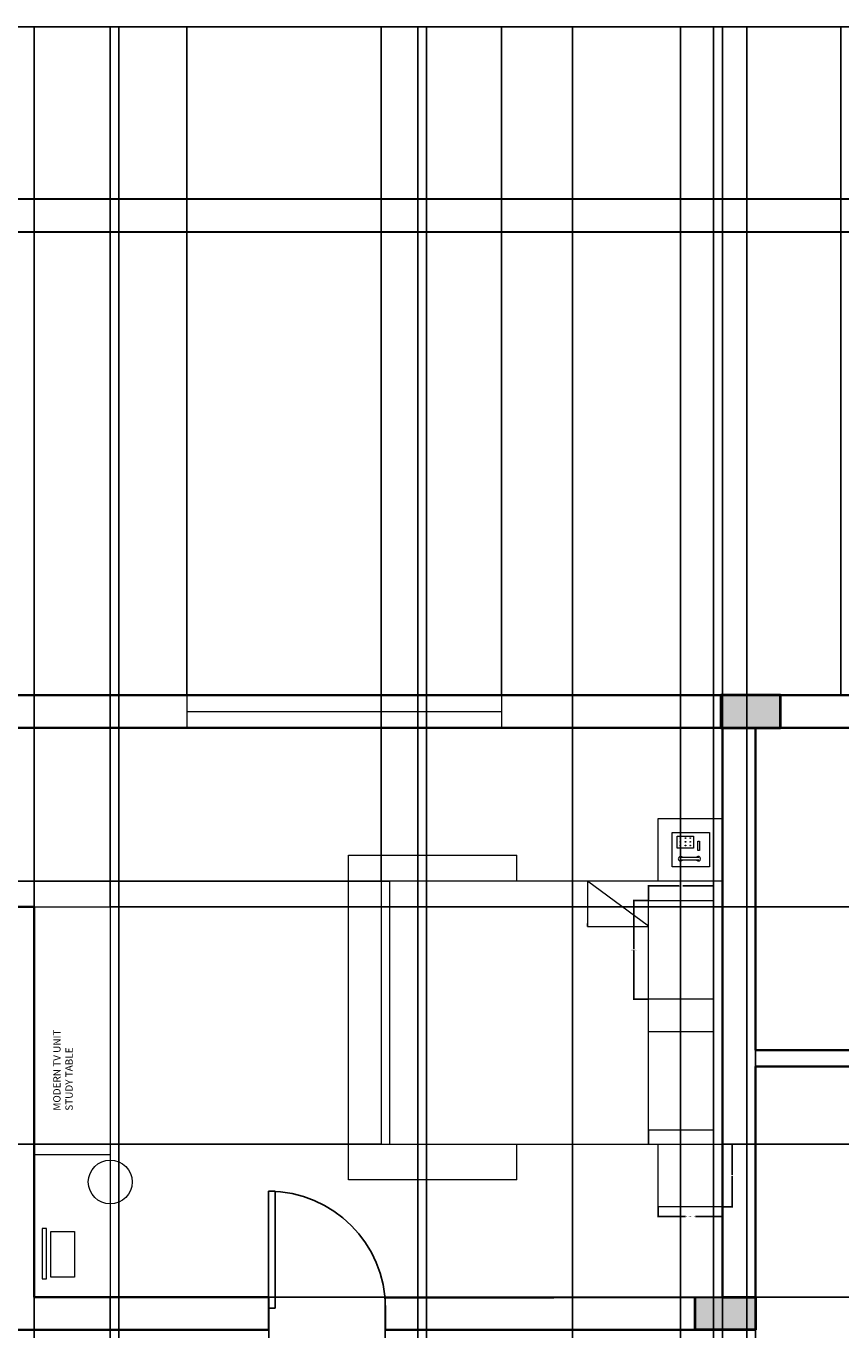
# Model space of a CAD drawing. Units: inches. Extents: x 1210 to 1836, y 84 to 1122.
# Tile 4 of 5: x 1353 to 1576, y 764 to 1122. Entities that reach past the tile are written whole.
import ezdxf

# ---------------------------------------------------------------- set-up
doc = ezdxf.new("R2010")
doc.units = ezdxf.units.IN
doc.header["$MEASUREMENT"] = 0
for name, color, linetype, lineweight in [('A-ANNO-DIMS', 2, 'Continuous', 18), ('A-ANNO-TEXT', 7, 'Continuous', 18), ('A-COLS', 7, 'Continuous', 40), ('A-COLS-PATT', 6, 'Continuous', 13), ('A-EQPM', 8, 'Continuous', 13), ('A-FURN', 9, 'Continuous', 18), ('A-FURN-FIXD', 32, 'Continuous', 18), ('A-GLAZ', 4, 'Continuous', 18), ('A-WALL', 7, 'Continuous', 35), ('C-PROP', 32, 'Continuous', 30), ('DOORS', 24, 'Continuous', 25)]:
    doc.layers.add(name, color=color, linetype=linetype, lineweight=lineweight)
doc.styles.get("Standard").update_dxf_attribs({"font": 'arial.ttf'})
doc.dimstyles.get("Standard").update_dxf_attribs({"dimtxt": 0.18, "dimasz": 0.18, "dimexe": 0.18, "dimexo": 0.0625, "dimgap": 0.09, "dimtad": 0, "dimtih": 1, "dimtoh": 1, "dimdec": 4, "dimzin": 0, "dimdsep": 46, "dimtxsty": 'Standard', "dimcen": 0.09, "dimadec": 0, "dimazin": 0, "dimtfac": 1, "dimtdec": 4, "dimtofl": 0, "dimtmove": 0, "dimatfit": 3, "dimfxl": 1, "dimtolj": 1, "dimtzin": 0, "dimarcsym": 0})

# ---------------------------------------------------------------- blocks, each defined once
blk = doc.blocks.new('*U6')
for p, q in [((0, 0), (0, -6)), ((32, 0), (32, -6))]:
    blk.add_line(p, q)
blk.add_lwpolyline([(0, 0), (0, 32), (1.75, 32), (1.75, 0)], close=True)
blk.add_arc((0, 0), 32, 0, 90)
blk = doc.blocks.new('PILLOW')
blk.add_lwpolyline([(0, 27), (17.76, 27), (17.76, 0), (0, 0)], close=True)
blk = doc.blocks.new('NIGHTSTAND')
blk.add_lwpolyline([(0, 17.21), (17.61, 17.21), (17.61, 0), (0, 0)], close=True)
blk = doc.blocks.new('STOOL-ROUND')
blk.add_circle((6, 6), 6)
blk = doc.blocks.new('*D16')
at = {"layer": 'A-ANNO-DIMS', "color": 0, "lineweight": -2, "transparency": 16777216}
for p, q in [((1522.97, 881.87), (1518.8, 881.87)), ((1518.98, 881.69), (1518.98, 868.55)), ((1518.98, 855.05), (1518.98, 868.19)), ((1522.97, 854.87), (1518.8, 854.87))]:
    blk.add_line(p, q, dxfattribs=at)
at = {"layer": 'A-ANNO-DIMS', "color": 0, "transparency": 16777216}
for points in [[(1518.95, 881.69), (1519.01, 881.69), (1518.98, 881.87)], [(1518.95, 855.05), (1519.01, 855.05), (1518.98, 854.87)]]:
    blk.add_solid(points, dxfattribs=at)
at = {"layer": 'Defpoints', "color": 0, "transparency": 16777216}
for p in [(1518.98, 881.87), (1523.03, 881.87), (1523.03, 854.87)]:
    blk.add_point(p, dxfattribs=at)
at = {"layer": 'A-ANNO-DIMS', "color": 0, "transparency": 16777216, "insert": (1518.98, 868.37), "char_height": 0.18, "attachment_point": 5}
blk.add_mtext('\\A1;PILLOW 27 TYP.', dxfattribs=at)
blk = doc.blocks.new('*D17')
at = {"layer": 'A-ANNO-DIMS', "color": 0, "lineweight": -2, "transparency": 16777216}
for p, q in [((1523.03, 881.93), (1523.03, 886.1)), ((1523.21, 885.92), (1531.4, 885.92)), ((1540.62, 885.92), (1532.43, 885.92)), ((1540.8, 881.93), (1540.8, 886.1))]:
    blk.add_line(p, q, dxfattribs=at)
at = {"layer": 'A-ANNO-DIMS', "color": 0, "transparency": 16777216}
for points in [[(1523.21, 885.95), (1523.21, 885.89), (1523.03, 885.92)], [(1540.62, 885.95), (1540.62, 885.89), (1540.8, 885.92)]]:
    blk.add_solid(points, dxfattribs=at)
at = {"layer": 'Defpoints', "color": 0, "transparency": 16777216}
for p in [(1540.8, 885.92), (1523.03, 881.87), (1540.8, 881.87)]:
    blk.add_point(p, dxfattribs=at)
at = {"layer": 'A-ANNO-DIMS', "color": 0, "transparency": 16777216, "insert": (1531.92, 885.92), "char_height": 0.18, "attachment_point": 5}
blk.add_mtext('\\A1;18 TYP.', dxfattribs=at)
blk = doc.blocks.new('*D18')
at = {"layer": 'A-ANNO-DIMS', "color": 0, "lineweight": -2, "transparency": 16777216}
for p, q in [((1525.71, 797.84), (1525.71, 795.08)), ((1543.32, 797.84), (1543.32, 795.08)), ((1525.89, 795.26), (1533.14, 795.26)), ((1543.14, 795.26), (1535.89, 795.26))]:
    blk.add_line(p, q, dxfattribs=at)
at = {"layer": 'A-ANNO-DIMS', "color": 0, "transparency": 16777216}
for points in [[(1525.89, 795.29), (1525.89, 795.23), (1525.71, 795.26)], [(1543.14, 795.29), (1543.14, 795.23), (1543.32, 795.26)]]:
    blk.add_solid(points, dxfattribs=at)
at = {"layer": 'Defpoints', "color": 0, "transparency": 16777216}
for p in [(1525.71, 797.91), (1543.32, 797.91), (1543.32, 795.26)]:
    blk.add_point(p, dxfattribs=at)
at = {"layer": 'A-ANNO-DIMS', "color": 0, "transparency": 16777216, "insert": (1534.52, 795.26), "char_height": 0.18, "attachment_point": 5}
blk.add_mtext('\\A1;NIGHTSTAND 18 TYP.', dxfattribs=at)
blk = doc.blocks.new('*D19')
at = {"layer": 'A-ANNO-DIMS', "color": 0, "lineweight": -2, "transparency": 16777216}
for p, q in [((1543.39, 815.12), (1546.15, 815.12)), ((1545.97, 814.94), (1545.97, 806.69)), ((1545.97, 798.09), (1545.97, 806.33)), ((1543.39, 797.91), (1546.15, 797.91))]:
    blk.add_line(p, q, dxfattribs=at)
at = {"layer": 'A-ANNO-DIMS', "color": 0, "transparency": 16777216}
for points in [[(1545.94, 814.94), (1546, 814.94), (1545.97, 815.12)], [(1545.94, 798.09), (1546, 798.09), (1545.97, 797.91)]]:
    blk.add_solid(points, dxfattribs=at)
at = {"layer": 'Defpoints', "color": 0, "transparency": 16777216}
for p in [(1543.32, 815.12), (1545.97, 815.12), (1543.32, 797.91)]:
    blk.add_point(p, dxfattribs=at)
at = {"layer": 'A-ANNO-DIMS', "color": 0, "transparency": 16777216, "insert": (1545.97, 806.51), "char_height": 0.18, "attachment_point": 5}
blk.add_mtext('\\A1;17 TYP.', dxfattribs=at)
blk = doc.blocks.new('*D22')
at = {"layer": 'A-ANNO-DIMS', "color": 0, "lineweight": -2, "transparency": 16777216}
for p, q in [((1257.32, 1074.28), (1257.32, 1121.57)), ((1257.5, 1121.39), (1522.55, 1121.39)), ((1788.14, 1121.39), (1523.1, 1121.39)), ((1788.32, 1074.28), (1788.32, 1121.57))]:
    blk.add_line(p, q, dxfattribs=at)
at = {"layer": 'A-ANNO-DIMS', "color": 0, "transparency": 16777216}
for points in [[(1257.5, 1121.42), (1257.5, 1121.36), (1257.32, 1121.39)], [(1788.14, 1121.42), (1788.14, 1121.36), (1788.32, 1121.39)]]:
    blk.add_solid(points, dxfattribs=at)
at = {"layer": 'Defpoints', "color": 0, "transparency": 16777216}
for p in [(1788.32, 1121.39), (1257.32, 1074.21), (1788.32, 1074.21)]:
    blk.add_point(p, dxfattribs=at)
at = {"layer": 'A-ANNO-DIMS', "color": 0, "transparency": 16777216, "insert": (1522.82, 1121.39), "char_height": 0.18, "attachment_point": 5}
blk.add_mtext('\\A1;531', dxfattribs=at)
blk = doc.blocks.new('*D36')
at = {"layer": 'A-ANNO-DIMS', "color": 0, "lineweight": -2, "transparency": 16777216}
for p, q in [((1552.32, 840.82), (1552.32, 83.86)), ((1661.32, 840.82), (1661.32, 83.86)), ((1552.5, 84.04), (1606.54, 84.04)), ((1661.14, 84.04), (1607.1, 84.04))]:
    blk.add_line(p, q, dxfattribs=at)
at = {"layer": 'A-ANNO-DIMS', "color": 0, "transparency": 16777216}
for points in [[(1552.5, 84.07), (1552.5, 84.01), (1552.32, 84.04)], [(1661.14, 84.07), (1661.14, 84.01), (1661.32, 84.04)]]:
    blk.add_solid(points, dxfattribs=at)
at = {"layer": 'Defpoints', "color": 0, "transparency": 16777216}
for p in [(1552.32, 840.89), (1661.32, 840.89), (1661.32, 84.04)]:
    blk.add_point(p, dxfattribs=at)
at = {"layer": 'A-ANNO-DIMS', "color": 0, "transparency": 16777216, "insert": (1606.82, 84.04), "char_height": 0.18, "attachment_point": 5}
blk.add_mtext('\\A1;109', dxfattribs=at)
blk = doc.blocks.new('*D39')
at = {"layer": 'A-ANNO-DIMS', "color": 0, "lineweight": -2, "transparency": 16777216}
for p, q in [((1354.82, 773.15), (1354.82, 83.86)), ((1543.32, 773.15), (1543.32, 83.86)), ((1355, 84.04), (1448.69, 84.04)), ((1543.14, 84.04), (1449.46, 84.04))]:
    blk.add_line(p, q, dxfattribs=at)
at = {"layer": 'A-ANNO-DIMS', "color": 0, "transparency": 16777216}
for points in [[(1355, 84.07), (1355, 84.01), (1354.82, 84.04)], [(1543.14, 84.07), (1543.14, 84.01), (1543.32, 84.04)]]:
    blk.add_solid(points, dxfattribs=at)
at = {"layer": 'Defpoints', "color": 0, "transparency": 16777216}
for p in [(1354.82, 773.21), (1543.32, 773.21), (1543.32, 84.04)]:
    blk.add_point(p, dxfattribs=at)
at = {"layer": 'A-ANNO-DIMS', "color": 0, "transparency": 16777216, "insert": (1449.07, 84.04), "char_height": 0.18, "attachment_point": 5}
blk.add_mtext('\\A1;188.5', dxfattribs=at)
blk = doc.blocks.new('*D42')
at = {"layer": 'A-ANNO-DIMS', "color": 0, "lineweight": -2, "transparency": 16777216}
for p, q in [((1354.82, 880.27), (1354.82, 1121.57)), ((1355, 1121.39), (1364.75, 1121.39)), ((1375.43, 1121.39), (1365.68, 1121.39)), ((1375.61, 880.27), (1375.61, 1121.57))]:
    blk.add_line(p, q, dxfattribs=at)
at = {"layer": 'A-ANNO-DIMS', "color": 0, "transparency": 16777216}
for points in [[(1355, 1121.42), (1355, 1121.36), (1354.82, 1121.39)], [(1375.43, 1121.42), (1375.43, 1121.36), (1375.61, 1121.39)]]:
    blk.add_solid(points, dxfattribs=at)
at = {"layer": 'Defpoints', "color": 0, "transparency": 16777216}
for p in [(1375.61, 1121.39), (1354.82, 880.21), (1375.61, 880.21)]:
    blk.add_point(p, dxfattribs=at)
at = {"layer": 'A-ANNO-DIMS', "color": 0, "transparency": 16777216, "insert": (1365.22, 1121.39), "char_height": 0.18, "attachment_point": 5}
blk.add_mtext('\\A1;20.786', dxfattribs=at)
blk = doc.blocks.new('*D43')
at = {"layer": 'A-ANNO-DIMS', "color": 0, "lineweight": -2, "transparency": 16777216}
for p, q in [((1375.67, 880.21), (1835.68, 880.21)), ((1835.5, 880.03), (1835.5, 826.9)), ((1835.5, 773.39), (1835.5, 826.53)), ((1375.67, 773.21), (1835.68, 773.21))]:
    blk.add_line(p, q, dxfattribs=at)
at = {"layer": 'A-ANNO-DIMS', "color": 0, "transparency": 16777216}
for points in [[(1835.47, 880.03), (1835.53, 880.03), (1835.5, 880.21)], [(1835.47, 773.39), (1835.53, 773.39), (1835.5, 773.21)]]:
    blk.add_solid(points, dxfattribs=at)
at = {"layer": 'Defpoints', "color": 0, "transparency": 16777216}
for p in [(1375.61, 880.21), (1835.5, 880.21), (1375.61, 773.21)]:
    blk.add_point(p, dxfattribs=at)
at = {"layer": 'A-ANNO-DIMS', "color": 0, "transparency": 16777216, "insert": (1835.5, 826.71), "char_height": 0.18, "attachment_point": 5}
blk.add_mtext('\\A1;107', dxfattribs=at)
blk = doc.blocks.new('*D44')
at = {"layer": 'A-ANNO-DIMS', "color": 0, "lineweight": -2, "transparency": 16777216}
for p, q in [((1449.85, 887.27), (1449.85, 1121.57)), ((1450.03, 1121.39), (1496.19, 1121.39)), ((1543.14, 1121.39), (1496.98, 1121.39)), ((1543.32, 904.47), (1543.32, 1121.57))]:
    blk.add_line(p, q, dxfattribs=at)
at = {"layer": 'A-ANNO-DIMS', "color": 0, "transparency": 16777216}
for points in [[(1450.03, 1121.42), (1450.03, 1121.36), (1449.85, 1121.39)], [(1543.14, 1121.42), (1543.14, 1121.36), (1543.32, 1121.39)]]:
    blk.add_solid(points, dxfattribs=at)
at = {"layer": 'Defpoints', "color": 0, "transparency": 16777216}
for p in [(1543.32, 1121.39), (1543.32, 904.41), (1449.85, 887.21)]:
    blk.add_point(p, dxfattribs=at)
at = {"layer": 'A-ANNO-DIMS', "color": 0, "transparency": 16777216, "insert": (1496.58, 1121.39), "char_height": 0.18, "attachment_point": 5}
blk.add_mtext('\\A1;93.48', dxfattribs=at)
blk = doc.blocks.new('*D45')
at = {"layer": 'A-ANNO-DIMS', "color": 0, "lineweight": -2, "transparency": 16777216}
for p, q in [((1449.78, 887.21), (1209.97, 887.21)), ((1210.15, 887.03), (1210.15, 851.34)), ((1210.15, 815.3), (1210.15, 850.98)), ((1449.78, 815.12), (1209.97, 815.12))]:
    blk.add_line(p, q, dxfattribs=at)
at = {"layer": 'A-ANNO-DIMS', "color": 0, "transparency": 16777216}
for points in [[(1210.12, 887.03), (1210.18, 887.03), (1210.15, 887.21)], [(1210.12, 815.3), (1210.18, 815.3), (1210.15, 815.12)]]:
    blk.add_solid(points, dxfattribs=at)
at = {"layer": 'Defpoints', "color": 0, "transparency": 16777216}
for p in [(1449.85, 887.21), (1210.15, 815.12), (1449.85, 815.12)]:
    blk.add_point(p, dxfattribs=at)
at = {"layer": 'A-ANNO-DIMS', "color": 0, "transparency": 16777216, "insert": (1210.15, 851.16), "char_height": 0.18, "attachment_point": 5}
blk.add_mtext('\\A1;72.1', dxfattribs=at)
blk = doc.blocks.new('*D46')
at = {"layer": 'A-ANNO-DIMS', "color": 0, "lineweight": -2, "transparency": 16777216}
for p, q in [((1543.39, 815.12), (1835.68, 815.12)), ((1835.5, 814.94), (1835.5, 794.35)), ((1835.5, 773.39), (1835.5, 793.98)), ((1543.39, 773.21), (1835.68, 773.21))]:
    blk.add_line(p, q, dxfattribs=at)
at = {"layer": 'A-ANNO-DIMS', "color": 0, "transparency": 16777216}
for points in [[(1835.47, 814.94), (1835.53, 814.94), (1835.5, 815.12)], [(1835.47, 773.39), (1835.53, 773.39), (1835.5, 773.21)]]:
    blk.add_solid(points, dxfattribs=at)
at = {"layer": 'Defpoints', "color": 0, "transparency": 16777216}
for p in [(1543.32, 815.12), (1543.32, 773.21), (1835.5, 773.21)]:
    blk.add_point(p, dxfattribs=at)
at = {"layer": 'A-ANNO-DIMS', "color": 0, "transparency": 16777216, "insert": (1835.5, 794.17), "char_height": 0.18, "attachment_point": 5}
blk.add_mtext('\\A1;41.9', dxfattribs=at)
blk = doc.blocks.new('*D47')
at = {"layer": 'A-ANNO-DIMS', "color": 0, "lineweight": -2, "transparency": 16777216}
for p, q in [((1375.61, 773.15), (1375.61, 83.86)), ((1419.01, 773.15), (1419.01, 83.86)), ((1375.79, 84.04), (1396.98, 84.04)), ((1418.83, 84.04), (1397.64, 84.04))]:
    blk.add_line(p, q, dxfattribs=at)
at = {"layer": 'A-ANNO-DIMS', "color": 0, "transparency": 16777216}
for points in [[(1375.79, 84.07), (1375.79, 84.01), (1375.61, 84.04)], [(1418.83, 84.07), (1418.83, 84.01), (1419.01, 84.04)]]:
    blk.add_solid(points, dxfattribs=at)
at = {"layer": 'Defpoints', "color": 0, "transparency": 16777216}
for p in [(1375.61, 773.21), (1419.01, 773.21), (1419.01, 84.04)]:
    blk.add_point(p, dxfattribs=at)
at = {"layer": 'A-ANNO-DIMS', "color": 0, "transparency": 16777216, "insert": (1397.31, 84.04), "char_height": 0.18, "attachment_point": 5}
blk.add_mtext('\\A1;43.4', dxfattribs=at)
blk = doc.blocks.new('*D48')
at = {"layer": 'A-ANNO-DIMS', "color": 0, "lineweight": -2, "transparency": 16777216}
for p, q in [((1419.01, 773.15), (1419.01, 83.86)), ((1450.89, 772.94), (1450.89, 83.86)), ((1419.19, 84.04), (1434.55, 84.04)), ((1450.71, 84.04), (1435.34, 84.04))]:
    blk.add_line(p, q, dxfattribs=at)
at = {"layer": 'A-ANNO-DIMS', "color": 0, "transparency": 16777216}
for points in [[(1419.19, 84.07), (1419.19, 84.01), (1419.01, 84.04)], [(1450.71, 84.07), (1450.71, 84.01), (1450.89, 84.04)]]:
    blk.add_solid(points, dxfattribs=at)
at = {"layer": 'Defpoints', "color": 0, "transparency": 16777216}
for p in [(1419.01, 773.21), (1450.89, 773), (1450.89, 84.04)]:
    blk.add_point(p, dxfattribs=at)
at = {"layer": 'A-ANNO-DIMS', "color": 0, "transparency": 16777216, "insert": (1434.95, 84.04), "char_height": 0.18, "attachment_point": 5}
blk.add_mtext('\\A1;31.88', dxfattribs=at)
blk = doc.blocks.new('*D51')
at = {"layer": 'A-ANNO-DIMS', "color": 0, "lineweight": -2, "transparency": 16777216}
for p, q in [((1333.21, 938.28), (1333.21, 1121.57)), ((1333.39, 1121.39), (1364.51, 1121.39)), ((1396.41, 1121.39), (1365.29, 1121.39)), ((1396.59, 938.28), (1396.59, 1121.57))]:
    blk.add_line(p, q, dxfattribs=at)
at = {"layer": 'A-ANNO-DIMS', "color": 0, "transparency": 16777216}
for points in [[(1333.39, 1121.42), (1333.39, 1121.36), (1333.21, 1121.39)], [(1396.41, 1121.42), (1396.41, 1121.36), (1396.59, 1121.39)]]:
    blk.add_solid(points, dxfattribs=at)
at = {"layer": 'Defpoints', "color": 0, "transparency": 16777216}
for p in [(1396.59, 1121.39), (1333.21, 938.21), (1396.59, 938.21)]:
    blk.add_point(p, dxfattribs=at)
at = {"layer": 'A-ANNO-DIMS', "color": 0, "transparency": 16777216, "insert": (1364.9, 1121.39), "char_height": 0.18, "attachment_point": 5}
blk.add_mtext('\\A1;63.39', dxfattribs=at)
blk = doc.blocks.new('*D52')
at = {"layer": 'A-ANNO-DIMS', "color": 0, "lineweight": -2, "transparency": 16777216}
for p, q in [((1396.59, 938.28), (1396.59, 1121.57)), ((1396.77, 1121.39), (1439.31, 1121.39)), ((1482.63, 1121.39), (1440.09, 1121.39)), ((1482.81, 938.28), (1482.81, 1121.57))]:
    blk.add_line(p, q, dxfattribs=at)
at = {"layer": 'A-ANNO-DIMS', "color": 0, "transparency": 16777216}
for points in [[(1396.77, 1121.42), (1396.77, 1121.36), (1396.59, 1121.39)], [(1482.63, 1121.42), (1482.63, 1121.36), (1482.81, 1121.39)]]:
    blk.add_solid(points, dxfattribs=at)
at = {"layer": 'Defpoints', "color": 0, "transparency": 16777216}
for p in [(1482.81, 1121.39), (1396.59, 938.21), (1482.81, 938.21)]:
    blk.add_point(p, dxfattribs=at)
at = {"layer": 'A-ANNO-DIMS', "color": 0, "transparency": 16777216, "insert": (1439.7, 1121.39), "char_height": 0.18, "attachment_point": 5}
blk.add_mtext('\\A1;86.22', dxfattribs=at)
blk = doc.blocks.new('*D53')
at = {"layer": 'A-ANNO-DIMS', "color": 0, "lineweight": -2, "transparency": 16777216}
for p, q in [((1482.81, 938.28), (1482.81, 1121.57)), ((1482.99, 1121.39), (1528.88, 1121.39)), ((1575.55, 1121.39), (1529.67, 1121.39)), ((1575.73, 938.28), (1575.73, 1121.57))]:
    blk.add_line(p, q, dxfattribs=at)
at = {"layer": 'A-ANNO-DIMS', "color": 0, "transparency": 16777216}
for points in [[(1482.99, 1121.42), (1482.99, 1121.36), (1482.81, 1121.39)], [(1575.55, 1121.42), (1575.55, 1121.36), (1575.73, 1121.39)]]:
    blk.add_solid(points, dxfattribs=at)
at = {"layer": 'Defpoints', "color": 0, "transparency": 16777216}
for p in [(1575.73, 1121.39), (1482.81, 938.21), (1575.73, 938.21)]:
    blk.add_point(p, dxfattribs=at)
at = {"layer": 'A-ANNO-DIMS', "color": 0, "transparency": 16777216, "insert": (1529.27, 1121.39), "char_height": 0.18, "attachment_point": 5}
blk.add_mtext('\\A1;92.92', dxfattribs=at)
blk = doc.blocks.new('*D59')
at = {"layer": 'A-ANNO-DIMS', "color": 0, "lineweight": -2, "transparency": 16777216}
for p, q in [((1459.82, 443.21), (1459.82, 1121.57)), ((1460, 1121.39), (1495.61, 1121.39)), ((1531.64, 1121.39), (1496.04, 1121.39)), ((1531.82, 443.21), (1531.82, 1121.57))]:
    blk.add_line(p, q, dxfattribs=at)
at = {"layer": 'A-ANNO-DIMS', "color": 0, "transparency": 16777216}
for points in [[(1460, 1121.42), (1460, 1121.36), (1459.82, 1121.39)], [(1531.64, 1121.42), (1531.64, 1121.36), (1531.82, 1121.39)]]:
    blk.add_solid(points, dxfattribs=at)
at = {"layer": 'Defpoints', "color": 0, "transparency": 16777216}
for p in [(1531.82, 1121.39), (1459.82, 443.15), (1531.82, 443.15)]:
    blk.add_point(p, dxfattribs=at)
at = {"layer": 'A-ANNO-DIMS', "color": 0, "transparency": 16777216, "insert": (1495.82, 1121.39), "char_height": 0.18, "attachment_point": 5}
blk.add_mtext('\\A1;72', dxfattribs=at)
blk = doc.blocks.new('*D60')
at = {"layer": 'A-ANNO-DIMS', "color": 0, "lineweight": -2, "transparency": 16777216}
for p, q in [((1540.82, 401.28), (1540.82, 1121.57)), ((1541, 1121.39), (1617.04, 1121.39)), ((1693.64, 1121.39), (1617.6, 1121.39)), ((1693.82, 401.28), (1693.82, 1121.57))]:
    blk.add_line(p, q, dxfattribs=at)
at = {"layer": 'A-ANNO-DIMS', "color": 0, "transparency": 16777216}
for points in [[(1541, 1121.42), (1541, 1121.36), (1540.82, 1121.39)], [(1693.64, 1121.42), (1693.64, 1121.36), (1693.82, 1121.39)]]:
    blk.add_solid(points, dxfattribs=at)
at = {"layer": 'Defpoints', "color": 0, "transparency": 16777216}
for p in [(1693.82, 1121.39), (1540.82, 401.21), (1693.82, 401.21)]:
    blk.add_point(p, dxfattribs=at)
at = {"layer": 'A-ANNO-DIMS', "color": 0, "transparency": 16777216, "insert": (1617.32, 1121.39), "char_height": 0.18, "attachment_point": 5}
blk.add_mtext('\\A1;153', dxfattribs=at)
blk = doc.blocks.new('*D65')
at = {"layer": 'A-ANNO-DIMS', "color": 0, "lineweight": -2, "transparency": 16777216}
for p, q in [((1549.93, 581.28), (1549.93, 1121.57)), ((1550.11, 1121.39), (1569.48, 1121.39)), ((1589.64, 1121.39), (1570.27, 1121.39)), ((1589.82, 581.28), (1589.82, 1121.57))]:
    blk.add_line(p, q, dxfattribs=at)
at = {"layer": 'A-ANNO-DIMS', "color": 0, "transparency": 16777216}
for points in [[(1550.11, 1121.42), (1550.11, 1121.36), (1549.93, 1121.39)], [(1589.64, 1121.42), (1589.64, 1121.36), (1589.82, 1121.39)]]:
    blk.add_solid(points, dxfattribs=at)
at = {"layer": 'Defpoints', "color": 0, "transparency": 16777216}
for p in [(1589.82, 1121.39), (1549.93, 581.21), (1589.82, 581.21)]:
    blk.add_point(p, dxfattribs=at)
at = {"layer": 'A-ANNO-DIMS', "color": 0, "transparency": 16777216, "insert": (1569.88, 1121.39), "char_height": 0.18, "attachment_point": 5}
blk.add_mtext('\\A1;39.89', dxfattribs=at)
blk = doc.blocks.new('*D73')
at = {"layer": 'A-ANNO-DIMS', "color": 0, "lineweight": -2, "transparency": 16777216}
for p, q in [((1302.49, 590.28), (1302.49, 1121.57)), ((1302.67, 1121.39), (1339.91, 1121.39)), ((1377.81, 1121.39), (1340.56, 1121.39)), ((1377.99, 590.28), (1377.99, 1121.57))]:
    blk.add_line(p, q, dxfattribs=at)
at = {"layer": 'A-ANNO-DIMS', "color": 0, "transparency": 16777216}
for points in [[(1302.67, 1121.42), (1302.67, 1121.36), (1302.49, 1121.39)], [(1377.81, 1121.42), (1377.81, 1121.36), (1377.99, 1121.39)]]:
    blk.add_solid(points, dxfattribs=at)
at = {"layer": 'Defpoints', "color": 0, "transparency": 16777216}
for p in [(1377.99, 1121.39), (1302.49, 590.21), (1377.99, 590.21)]:
    blk.add_point(p, dxfattribs=at)
at = {"layer": 'A-ANNO-DIMS', "color": 0, "transparency": 16777216, "insert": (1340.24, 1121.39), "char_height": 0.18, "attachment_point": 5}
blk.add_mtext('\\A1;75.5', dxfattribs=at)
blk = doc.blocks.new('*D76')
at = {"layer": 'A-ANNO-DIMS', "color": 0, "lineweight": -2, "transparency": 16777216}
for p, q in [((1462.25, 528.78), (1462.25, 1121.57)), ((1462.43, 1121.39), (1482.03, 1121.39)), ((1502.07, 1121.39), (1482.47, 1121.39)), ((1502.25, 528.78), (1502.25, 1121.57))]:
    blk.add_line(p, q, dxfattribs=at)
at = {"layer": 'A-ANNO-DIMS', "color": 0, "transparency": 16777216}
for points in [[(1462.43, 1121.42), (1462.43, 1121.36), (1462.25, 1121.39)], [(1502.07, 1121.42), (1502.07, 1121.36), (1502.25, 1121.39)]]:
    blk.add_solid(points, dxfattribs=at)
at = {"layer": 'Defpoints', "color": 0, "transparency": 16777216}
for p in [(1502.25, 1121.39), (1462.25, 528.71), (1502.25, 528.71)]:
    blk.add_point(p, dxfattribs=at)
at = {"layer": 'A-ANNO-DIMS', "color": 0, "transparency": 16777216, "insert": (1482.25, 1121.39), "char_height": 0.18, "attachment_point": 5}
blk.add_mtext('\\A1;40', dxfattribs=at)

msp = doc.modelspace()

# ---------------------------------------------------------------- hatches: boundary and pattern name
at = {"layer": 'A-COLS-PATT'}
h = msp.add_hatch(color=256, dxfattribs=at)
h.dxf.hatch_style = 1
h.paths.add_polyline_path([(1266.3239, 938.214), (1257.3239, 938.214), (1257.3239, 929.4573), (1257.3239, 923.2025), (1266.3239, 923.2025)])
h.paths.add_polyline_path([(1350.3239, 929.214), (1350.3239, 938.214), (1339.1886, 938.214), (1339.1886, 929.214)])
h.paths.add_polyline_path([(1559.1961, 929.214), (1559.1961, 938.214), (1542.8626, 938.214), (1542.8626, 929.214), (1543.3239, 929.214)])
h.paths.add_polyline_path([(1771.5139, 938.214), (1771.5139, 929.214), (1788.3239, 929.214), (1788.3239, 938.214)])
h.paths.add_polyline_path([(1788.3239, 764.214), (1788.3239, 773.214), (1775.2119, 773.214), (1775.2119, 764.214)])
h.paths.add_polyline_path([(1552.3239, 764.214), (1552.3239, 773.214), (1543.3239, 773.214), (1535.8494, 773.197), (1535.8494, 764.214)])
h.paths.add_polyline_path([(1275.5217, 782.2138), (1272.7843, 782.2138), (1266.3239, 782.2138), (1266.3239, 764.214), (1275.5217, 764.214)])
h.paths.add_polyline_path([(1350.2372, 764.214), (1350.3239, 773.214), (1343.6352, 773.214), (1343.6352, 764.214)])
h.paths.add_polyline_path([(1257.3239, 570.3846), (1266.3239, 570.3846), (1266.3239, 590.214), (1257.3239, 590.214)])
h.paths.add_polyline_path([(1450.8239, 572.5809), (1459.8239, 572.5809), (1459.8239, 590.214), (1458.3239, 590.214), (1450.8239, 590.214)])
h.paths.add_polyline_path([(1531.8239, 572.5809), (1540.8239, 572.5809), (1540.8239, 590.214), (1531.8239, 590.214)])
h.paths.add_polyline_path([(1450.8239, 392.214), (1459.8239, 392.214), (1459.8239, 401.214), (1459.8239, 408.7866), (1450.8239, 408.7866)])
h.paths.add_polyline_path([(1531.8239, 392.214), (1540.8239, 392.214), (1540.8239, 401.214), (1540.8239, 408.7866), (1531.8239, 408.7866)])
h.paths.add_polyline_path([(1682.9725, 401.214), (1682.9725, 392.214), (1698.3239, 392.214), (1698.3239, 401.214), (1693.8239, 401.214)])
h.paths.add_polyline_path([(1774.197, 350.714), (1779.3239, 350.714), (1788.3239, 350.714), (1788.3239, 359.714), (1779.3239, 359.714), (1774.197, 359.714)])
h.paths.add_polyline_path([(1779.3239, 590.214), (1775.4485, 590.214), (1775.4485, 581.214), (1779.3239, 581.214), (1788.3239, 581.214), (1788.3239, 590.214)])

# ---------------------------------------------------------------- linework, layer by layer
at = {"layer": 'A-COLS'}
for p, q in [((1559.1961, 938.214), (1542.8626, 938.214)), ((1542.8626, 938.214), (1542.8626, 929.214)), ((1559.1961, 929.214), (1559.1961, 938.214)), ((1542.8626, 929.214), (1543.3239, 929.214)), ((1543.3239, 929.214), (1559.1961, 929.214)), ((1535.8494, 764.214), (1535.8494, 773.214)), ((1543.3239, 773.214), (1552.3239, 773.214)), ((1552.3239, 773.214), (1552.3239, 764.214)), ((1552.3239, 764.214), (1535.8494, 764.214))]:
    msp.add_line(p, q, dxfattribs=at)
at = {"layer": 'A-EQPM'}
for p, q in [((1357.014, 791.978), (1357.014, 778.183)), ((1358.1894, 791.978), (1357.014, 791.978)), ((1358.1894, 778.183), (1358.1894, 791.978)), ((1357.014, 778.183), (1357.014, 778.183)), ((1357.014, 778.183), (1358.1894, 778.183))]:
    msp.add_line(p, q, dxfattribs=at)
for points in [[(1529.5354, 900.5446), (1539.7767, 900.5446), (1539.7767, 891.1454), (1529.5354, 891.1454)], [(1530.8977, 899.5783), (1535.3407, 899.5783), (1535.3407, 896.2074), (1530.8977, 896.2074)], [(1536.5918, 898.2033), (1536.9849, 898.2033), (1536.9849, 895.5778), (1536.5918, 895.5778)], [(1359.3767, 791.2078), (1365.7929, 791.2078), (1365.7929, 778.6806), (1359.3767, 778.6806)]]:
    msp.add_lwpolyline(points, close=True, dxfattribs=at)
for points in [[(1531.7124, 893.797), (1536.7807, 893.797)], [(1536.7807, 892.9623), (1531.7124, 892.9623)]]:
    msp.add_lwpolyline(points, dxfattribs=at)
for centre in [(1531.7709, 899.0336), (1531.7709, 897.9875), (1531.7709, 896.9878), (1533.1669, 899.0336), (1533.1669, 897.9875), (1533.1669, 896.9878), (1534.4931, 899.0336), (1534.4931, 897.9875), (1534.4931, 896.9878)]:
    msp.add_circle(centre, 0.0931, dxfattribs=at)
for centre, start, end in [((1531.8423, 893.3704), 42.323457, 319.906339), ((1536.6878, 893.3704), 220.093661, 137.676543)]:
    msp.add_arc(centre, 0.6337, start, end, dxfattribs=at)
at = {"layer": 'A-FURN'}
for p, q in [((1440.8449, 805.3673), (1440.8449, 894.3092)), ((1440.8449, 894.3092), (1486.9727, 894.3092)), ((1486.9727, 887.2124), (1486.9727, 894.3092)), ((1543.3239, 887.2124), (1449.8451, 887.2124)), ((1449.8451, 887.2124), (1449.8451, 815.1167)), ((1449.8451, 887.2124), (1452.0834, 887.2124)), ((1452.0834, 887.2124), (1452.0834, 815.1167)), ((1523.0345, 874.9178), (1506.2982, 887.2124)), ((1506.2982, 887.2124), (1506.2982, 874.7864)), ((1543.3239, 815.1167), (1543.3239, 887.2124)), ((1506.2982, 874.7864), (1506.2982, 875.601)), ((1506.2982, 875.601), (1506.2982, 874.7864)), ((1506.2982, 874.7864), (1523.0345, 874.7864)), ((1523.0345, 815.1167), (1523.0345, 874.9178)), ((1523.0345, 818.9983), (1523.0345, 815.1167)), ((1449.8451, 815.1167), (1543.3239, 815.1167)), ((1486.9727, 805.3673), (1486.9727, 815.1167)), ((1444.8749, 805.3673), (1440.8449, 805.3673)), ((1486.9727, 805.3673), (1444.8749, 805.3673))]:
    msp.add_line(p, q, dxfattribs=at)
at = {"layer": 'A-FURN-FIXD'}
for p, q in [((1354.8239, 880.2123), (1375.6096, 880.2123)), ((1375.6096, 880.2123), (1375.6096, 773.214)), ((1354.8239, 812.2728), (1375.6096, 812.2728))]:
    msp.add_line(p, q, dxfattribs=at)
at = {"layer": 'A-GLAZ'}
for p, q in [((1396.5935, 938.214), (1396.5935, 929.214)), ((1482.8101, 938.214), (1482.8101, 929.214)), ((1396.5935, 933.714), (1482.8101, 933.714))]:
    msp.add_line(p, q, dxfattribs=at)
at = {"layer": 'A-WALL'}
for p, q in [((1266.3239, 938.214), (1673.9914, 938.214)), ((1350.3239, 938.214), (1396.5935, 938.214)), ((1354.8239, 929.214), (1333.2056, 929.214)), ((1354.8239, 929.214), (1543.3239, 929.214)), ((1543.3239, 773.214), (1543.3239, 929.214)), ((1552.3239, 929.214), (1661.3239, 929.214)), ((1552.3239, 840.8861), (1552.3239, 929.214)), ((1350.3239, 880.2123), (1354.8239, 880.2123)), ((1354.8239, 773.214), (1354.8239, 880.2123)), ((1552.3239, 840.8861), (1615.4388, 840.8861)), ((1552.3239, 773.214), (1552.3239, 836.3861)), ((1615.4388, 836.3861), (1552.3239, 836.3861)), ((1354.8239, 773.214), (1419.0081, 773.214)), ((1450.8864, 773.0031), (1543.3239, 773.214)), ((1552.3239, 773.214), (1552.3239, 764.214)), ((1266.3239, 764.214), (1419.0081, 764.214)), ((1451.0081, 764.214), (1552.3239, 764.214))]:
    msp.add_line(p, q, dxfattribs=at)
at = {"layer": 'C-PROP'}
for p, q in [((1257.3239, 1074.214), (1788.3239, 1074.214)), ((1266.3239, 1065.214), (1779.3239, 1065.214))]:
    msp.add_line(p, q, dxfattribs=at)

# ---------------------------------------------------------------- block references
at = {"layer": 'A-FURN'}
for name, p in [('NIGHTSTAND', (1525.711, 887.1987)), ('PILLOW', (1523.035, 854.87)), ('PILLOW', (1523.035, 818.9983)), ('NIGHTSTAND', (1525.711, 797.905)), ('STOOL-ROUND', (1369.6118, 798.7644))]:
    msp.add_blockref(name, p, dxfattribs=at)
at = {"layer": 'DOORS'}
msp.add_blockref('*U6', (1419.0081, 770.214), dxfattribs=at)

# ---------------------------------------------------------------- texts
at = {"layer": 'A-ANNO-TEXT', "insert": (1360.006, 824.2966), "char_height": 2, "attachment_point": 1, "rotation": 90}
msp.add_mtext_dynamic_manual_height_columns('{MODERN TV UNIT\\PSTUDY TABLE}', width=293.611423, gutter_width=1, heights=[0], dxfattribs=at)

# ---------------------------------------------------------------- dimensions: what is measured, and where the dimension line sits
at = {"layer": 'A-ANNO-DIMS'}
for base, p1, p2, override, picture, middle in [((1788.3239, 1121.389), (1257.3239, 1074.214), (1788.3239, 1074.214), {"dimdec": 0, "dimlfac": 1, "dimrnd": 0, "dimzin": 0, "dimdsep": 46, "dimlunit": 2}, '*D22', (1522.8239, 1121.389)), ((1377.9853, 1121.389), (1302.4894, 590.214), (1377.9853, 590.214), {"dimdec": 1, "dimlfac": 1, "dimrnd": 0, "dimzin": 0, "dimdsep": 46, "dimlunit": 2}, '*D73', (1340.2374, 1121.389)), ((1396.5935, 1121.389), (1333.2056, 938.214), (1396.5935, 938.214), {"dimdec": 2, "dimlfac": 1, "dimrnd": 0, "dimzin": 0, "dimdsep": 46, "dimlunit": 2}, '*D51', (1364.8996, 1121.389)), ((1375.6096, 1121.389), (1354.8239, 880.2123), (1375.6096, 880.2123), {"dimdec": 3, "dimlfac": 1, "dimrnd": 0, "dimzin": 0, "dimdsep": 46, "dimlunit": 2}, '*D42', (1365.2167, 1121.389)), ((1482.8101, 1121.389), (1396.5935, 938.214), (1482.8101, 938.214), {"dimdec": 2, "dimlfac": 1, "dimrnd": 0, "dimzin": 0, "dimdsep": 46, "dimlunit": 2}, '*D52', (1439.7018, 1121.389)), ((1543.3239, 1121.389), (1449.8451, 887.2124), (1543.3239, 904.4104), {"dimdec": 2, "dimlfac": 1, "dimrnd": 0, "dimzin": 0, "dimdsep": 46, "dimlunit": 2}, '*D44', (1496.5845, 1121.389)), ((1531.8239, 1121.389), (1459.8239, 443.1518), (1531.8239, 443.1518), {"dimdec": 0, "dimlfac": 1, "dimrnd": 0, "dimzin": 0, "dimdsep": 46, "dimlunit": 2}, '*D59', (1495.8239, 1121.389)), ((1502.2498, 1121.389), (1462.2498, 528.714), (1502.2498, 528.714), {"dimdec": 0, "dimlfac": 1, "dimrnd": 0, "dimzin": 0, "dimdsep": 46, "dimlunit": 2}, '*D76', (1482.2498, 1121.389)), ((1575.7346, 1121.389), (1482.8101, 938.214), (1575.7346, 938.214), {"dimdec": 2, "dimlfac": 1, "dimrnd": 0, "dimzin": 0, "dimdsep": 46, "dimlunit": 2}, '*D53', (1529.2723, 1121.389)), ((1693.8239, 1121.389), (1540.8239, 401.214), (1693.8239, 401.214), {"dimdec": 0, "dimlfac": 1, "dimrnd": 0, "dimzin": 0, "dimdsep": 46, "dimlunit": 2}, '*D60', (1617.3239, 1121.389)), ((1589.8208, 1121.389), (1549.9335, 581.214), (1589.8208, 581.214), {"dimdec": 2, "dimlfac": 1, "dimrnd": 0, "dimzin": 0, "dimdsep": 46, "dimlunit": 2}, '*D65', (1569.8772, 1121.389)), ((1661.3239, 84.039), (1552.3239, 840.8861), (1661.3239, 840.8861), {"dimdec": 0, "dimlfac": 1, "dimrnd": 0, "dimzin": 0, "dimdsep": 46, "dimlunit": 2}, '*D36', (1606.8239, 84.039)), ((1543.3239, 84.039), (1354.8239, 773.214), (1543.3239, 773.214), {"dimdec": 1, "dimlfac": 1, "dimrnd": 0, "dimzin": 0, "dimdsep": 46, "dimlunit": 2}, '*D39', (1449.0739, 84.039)), ((1419.0081, 84.039), (1375.6096, 773.214), (1419.0081, 773.214), {"dimdec": 1, "dimlfac": 1, "dimrnd": 0, "dimzin": 0, "dimdsep": 46, "dimlunit": 2}, '*D47', (1397.3088, 84.039)), ((1450.8864, 84.039), (1419.0081, 773.214), (1450.8864, 773.0031), {"dimdec": 2, "dimlfac": 1, "dimrnd": 0, "dimzin": 0, "dimdsep": 46, "dimlunit": 2}, '*D48', (1434.9472, 84.039))]:
    dim = msp.add_linear_dim(base=base, p1=p1, p2=p2, dimstyle='Standard', override=override, dxfattribs=at)
    dim.commit()
    dim.dimension.update_dxf_attribs({"geometry": picture, "text_midpoint": middle})
for base, p1, p2, override, picture, middle in [((1210.1489, 815.1167), (1449.8451, 887.2124), (1449.8451, 815.1167), {"dimdec": 1, "dimlfac": 1, "dimrnd": 0, "dimzin": 0, "dimdsep": 46, "dimlunit": 2}, '*D45', (1210.1489, 851.1646)), ((1835.4989, 880.2123), (1375.6096, 773.214), (1375.6096, 880.2123), {"dimdec": 0, "dimlfac": 1, "dimrnd": 0, "dimzin": 0, "dimdsep": 46, "dimlunit": 2}, '*D43', (1835.4989, 826.7132)), ((1835.4989, 773.214), (1543.3239, 815.1167), (1543.3239, 773.214), {"dimdec": 1, "dimlfac": 1, "dimrnd": 0, "dimzin": 0, "dimdsep": 46, "dimlunit": 2}, '*D46', (1835.4989, 794.1654))]:
    dim = msp.add_linear_dim(base=base, p1=p1, p2=p2, angle=90, dimstyle='Standard', override=override, dxfattribs=at)
    dim.commit()
    dim.dimension.update_dxf_attribs({"geometry": picture, "text_midpoint": middle})
for base, p1, p2, text, picture, middle in [((1540.7959, 885.9179), (1523.0345, 881.8682), (1540.7959, 881.8682), '<> TYP.', '*D17', (1531.9152, 885.9179)), ((1543.3239, 795.2631), (1525.7112, 797.905), (1543.3239, 797.905), 'NIGHTSTAND <> TYP.', '*D18', (1534.5176, 795.2631))]:
    dim = msp.add_linear_dim(base=base, p1=p1, p2=p2, text=text, dimstyle='Standard', override={"dimdec": 0, "dimlfac": 1, "dimrnd": 0, "dimzin": 0, "dimdsep": 46, "dimlunit": 2}, dxfattribs=at)
    dim.commit()
    dim.dimension.update_dxf_attribs({"geometry": picture, "text_midpoint": middle})
for base, p1, p2, text, picture, middle in [((1518.9848, 881.8682), (1523.0345, 854.87), (1523.0345, 881.8682), 'PILLOW <> TYP.', '*D16', (1518.9848, 868.3691)), ((1545.9658, 815.1167), (1543.3239, 797.905), (1543.3239, 815.1167), '<> TYP.', '*D19', (1545.9658, 806.5109))]:
    dim = msp.add_linear_dim(base=base, p1=p1, p2=p2, angle=90, text=text, dimstyle='Standard', override={"dimdec": 0, "dimlfac": 1, "dimrnd": 0, "dimzin": 0, "dimdsep": 46, "dimlunit": 2}, dxfattribs=at)
    dim.commit()
    dim.dimension.update_dxf_attribs({"geometry": picture, "text_midpoint": middle})

doc.saveas('drawing.dxf')
